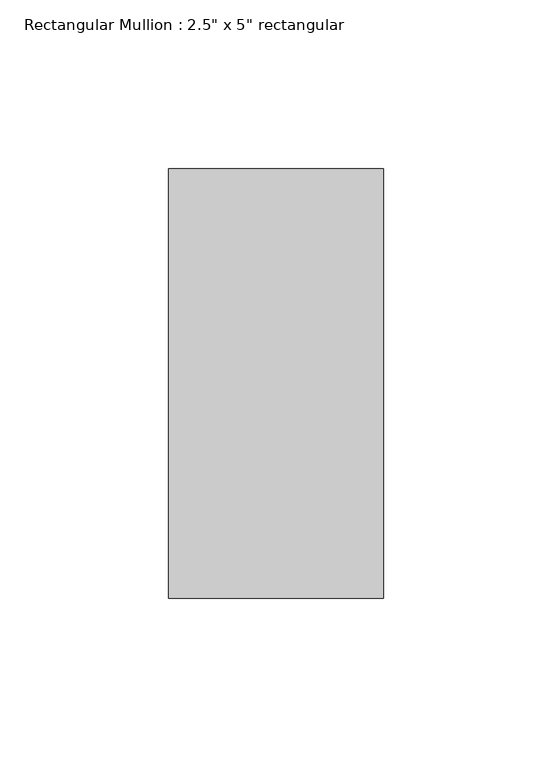
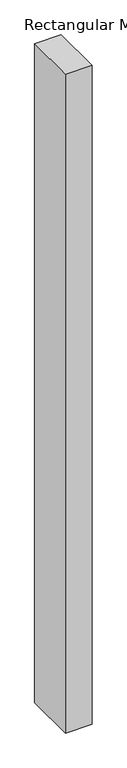
"""IFC4 building model written with IfcOpenShell, lengths in millimetres: member geometry."""

from ifc_helpers import new_model, si_unit, frame, origin, place, context, project, spatial, polyline, outline, extrude, source, transform, mapped, element, save


def member_049ba45b(model_context):
    return source(origin(), model_context, "Body", "SweptSolid", [
        extrude(outline(polyline([(31.75, 63.5), (31.75, -63.5), (-31.75, -63.5), (-31.75, 63.5), (31.75, 63.5)])), frame((0.0, 0.0, -1665.3902237), z_axis=(0.0, 0.0, 1.0), x_axis=(1.0, 0.0, 0.0)), (0.0, 0.0, 1.0), 1665.3902237),
    ])


if __name__ == "__main__":
    model = new_model("IFC4")
    model_context = context("Model", 3, world=origin())
    ifc_project = project(units=[si_unit("LENGTHUNIT", "METRE", prefix="MILLI")], contexts=[model_context])
    site = spatial("IfcSite", under=ifc_project)
    building = spatial("IfcBuilding", under=site)
    placement = place(None, origin())
    member_shape = member_049ba45b(model_context)
    element("IfcMember", 1, ObjectType="Rectangular Mullion : 2.5\" x 5\" rectangular", at=placement, inside=building, context=model_context, shape_type="MappedRepresentation", body=[
        mapped(member_shape, transform((0.0, 0.0, 0.0), x_axis=(1.0, 0.0, 0.0), y_axis=(0.0, 1.0, 0.0), z_axis=(0.0, 0.0, 1.0))),
    ])
    save(model, "model.ifc")

# Revit data of these elements
# Type "Rectangular Mullion : 2.5\" x 5\" rectangular"
#   built-in parameter 1007304 = 0.416667 (stored number, unit not read)
#   built-in parameter 1007301 = 0.104167 (stored number, unit not read)
#   built-in parameter 1007300 = 0.104167 (stored number, unit not read)
# Element 1 (IfcMember, "Rectangular Mullion : 2.5\" x 5\" rectangular")
#   Materials on its faces: "Aluminum"
# Materials
#   "Aluminum": class "Metal", colour RGB 247 247 247, transparency 0, Description = "Aluminum 6061", Cost = 0
